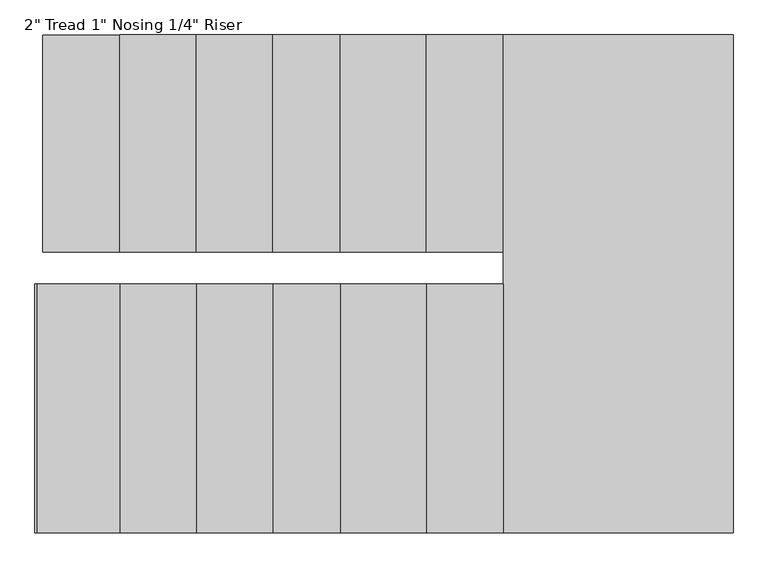
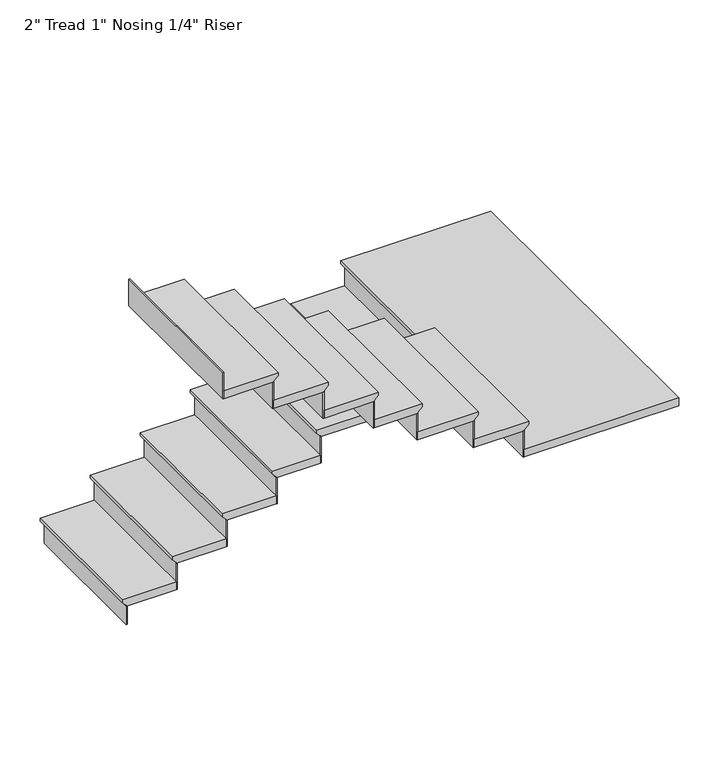
"""IFC4 building model written with IfcOpenShell, lengths in millimetres: stair flight geometry."""

from ifc_helpers import new_model, si_unit, origin, place, context, project, spatial, faceted_brep, source, transform, mapped, element, save


def stair_flight_0b56c5f1(model_context):
    return source(origin(), model_context, "Body", "Brep", [
        faceted_brep([(-879.540747, -2928.9064015, 150.2833333), (-879.540747, -2928.9064015, 169.3333333), (-879.540747, -2065.3064015, 169.3333333), (-879.540747, -2065.3064015, 150.2833333), (-854.140747, -2928.9064015, 124.8833333), (-854.140747, -2065.3064015, 124.8833333), (-549.340747, -2928.9064015, 169.3333333), (-549.340747, -2065.3064015, 169.3333333), (-854.140747, -2065.3064015, 118.5333333), (-549.340747, -2065.3064015, 118.5333333), (-549.340747, -2928.9064015, 118.5333333), (-854.140747, -2928.9064015, 118.5333333)], [[[0, 1, 2, 3]], [[4, 0, 3, 5]], [[2, 1, 6, 7]], [[8, 9, 10, 11]], [[2, 7, 9, 8, 5, 3]], [[8, 11, 4, 5]], [[6, 1, 0, 4, 11, 10]], [[7, 6, 10, 9]]]),
        faceted_brep([(-854.140747, -2928.9064015, 118.5333333), (-854.140747, -2928.9064015, 0.0), (-847.790747, -2928.9064015, 0.0), (-847.790747, -2928.9064015, 118.5333333), (-854.140747, -2065.3064015, 118.5333333), (-847.790747, -2065.3064015, 118.5333333), (-847.790747, -2065.3064015, 0.0), (-854.140747, -2065.3064015, 0.0)], [[[0, 1, 2, 3]], [[4, 5, 6, 7]], [[1, 0, 4, 7]], [[2, 1, 7, 6]], [[3, 2, 6, 5]], [[0, 3, 5, 4]]]),
        faceted_brep([(-549.340747, -2928.9064015, 287.8666667), (-549.340747, -2928.9064015, 118.5333333), (-542.990747, -2928.9064015, 118.5333333), (-542.990747, -2928.9064015, 287.8666667), (-549.340747, -2065.3064015, 287.8666667), (-542.990747, -2065.3064015, 287.8666667), (-542.990747, -2065.3064015, 118.5333333), (-549.340747, -2065.3064015, 118.5333333)], [[[0, 1, 2, 3]], [[4, 5, 6, 7]], [[1, 0, 4, 7]], [[2, 1, 7, 6]], [[3, 2, 6, 5]], [[0, 3, 5, 4]]]),
        faceted_brep([(-574.740747, -2065.3064015, 338.6666667), (-574.740747, -2928.9064015, 338.6666667), (-244.540747, -2928.9064015, 338.6666667), (-244.540747, -2065.3064015, 338.6666667), (-549.340747, -2065.3064015, 287.8666667), (-244.540747, -2065.3064015, 287.8666667), (-244.540747, -2928.9064015, 287.8666667), (-549.340747, -2928.9064015, 287.8666667), (-549.340747, -2065.3064015, 294.2166667), (-574.740747, -2065.3064015, 319.6166667), (-549.340747, -2928.9064015, 294.2166667), (-574.740747, -2928.9064015, 319.6166667)], [[[0, 1, 2, 3]], [[4, 5, 6, 7]], [[0, 3, 5, 4, 8, 9]], [[4, 7, 10, 8]], [[2, 1, 11, 10, 7, 6]], [[3, 2, 6, 5]], [[11, 1, 0, 9]], [[10, 11, 9, 8]]]),
        faceted_brep([(-244.540747, -2928.9064015, 457.2), (-244.540747, -2928.9064015, 287.8666667), (-238.190747, -2928.9064015, 287.8666667), (-238.190747, -2928.9064015, 457.2), (-244.540747, -2065.3064015, 457.2), (-238.190747, -2065.3064015, 457.2), (-238.190747, -2065.3064015, 287.8666667), (-244.540747, -2065.3064015, 287.8666667)], [[[0, 1, 2, 3]], [[4, 5, 6, 7]], [[1, 0, 4, 7]], [[2, 1, 7, 6]], [[3, 2, 6, 5]], [[0, 3, 5, 4]]]),
        faceted_brep([(-269.940747, -2065.3064015, 508.0), (-269.940747, -2928.9064015, 508.0), (60.259253, -2928.9064015, 508.0), (60.259253, -2065.3064015, 508.0), (-244.540747, -2065.3064015, 457.2), (60.259253, -2065.3064015, 457.2), (60.259253, -2928.9064015, 457.2), (-244.540747, -2928.9064015, 457.2), (-244.540747, -2065.3064015, 463.55), (-269.940747, -2065.3064015, 488.95), (-244.540747, -2928.9064015, 463.55), (-269.940747, -2928.9064015, 488.95)], [[[0, 1, 2, 3]], [[4, 5, 6, 7]], [[0, 3, 5, 4, 8, 9]], [[4, 7, 10, 8]], [[2, 1, 11, 10, 7, 6]], [[3, 2, 6, 5]], [[11, 1, 0, 9]], [[10, 11, 9, 8]]]),
        faceted_brep([(60.259253, -2928.9064015, 626.5333333), (60.259253, -2928.9064015, 457.2), (66.609253, -2928.9064015, 457.2), (66.609253, -2928.9064015, 626.5333333), (60.259253, -2065.3064015, 626.5333333), (66.609253, -2065.3064015, 626.5333333), (66.609253, -2065.3064015, 457.2), (60.259253, -2065.3064015, 457.2)], [[[0, 1, 2, 3]], [[4, 5, 6, 7]], [[1, 0, 4, 7]], [[2, 1, 7, 6]], [[3, 2, 6, 5]], [[0, 3, 5, 4]]]),
        faceted_brep([(34.859253, -2065.3064015, 677.3333333), (34.859253, -2928.9064015, 677.3333333), (326.959253, -2928.9064015, 677.3333333), (326.959253, -2065.3064015, 677.3333333), (60.259253, -2065.3064015, 626.5333333), (326.959253, -2065.3064015, 626.5333333), (326.959253, -2928.9064015, 626.5333333), (60.259253, -2928.9064015, 626.5333333), (60.259253, -2065.3064015, 632.8833333), (34.859253, -2065.3064015, 658.2833333), (60.259253, -2928.9064015, 632.8833333), (34.859253, -2928.9064015, 658.2833333)], [[[0, 1, 2, 3]], [[4, 5, 6, 7]], [[0, 3, 5, 4, 8, 9]], [[4, 7, 10, 8]], [[2, 1, 11, 10, 7, 6]], [[3, 2, 6, 5]], [[11, 1, 0, 9]], [[10, 11, 9, 8]]]),
        faceted_brep([(326.959253, -2928.9064015, 795.8666667), (326.959253, -2928.9064015, 626.5333333), (333.309253, -2928.9064015, 626.5333333), (333.309253, -2928.9064015, 795.8666667), (326.959253, -2065.3064015, 795.8666667), (333.309253, -2065.3064015, 795.8666667), (333.309253, -2065.3064015, 626.5333333), (326.959253, -2065.3064015, 626.5333333)], [[[0, 1, 2, 3]], [[4, 5, 6, 7]], [[1, 0, 4, 7]], [[2, 1, 7, 6]], [[3, 2, 6, 5]], [[0, 3, 5, 4]]]),
        faceted_brep([(301.559253, -2065.3064015, 846.6666667), (301.559253, -2928.9064015, 846.6666667), (669.859253, -2928.9064015, 846.6666667), (669.859253, -2065.3064015, 846.6666667), (326.959253, -2065.3064015, 795.8666667), (669.859253, -2065.3064015, 795.8666667), (669.859253, -2928.9064015, 795.8666667), (326.959253, -2928.9064015, 795.8666667), (326.959253, -2065.3064015, 802.2166667), (301.559253, -2065.3064015, 827.6166667), (326.959253, -2928.9064015, 802.2166667), (301.559253, -2928.9064015, 827.6166667)], [[[0, 1, 2, 3]], [[4, 5, 6, 7]], [[0, 3, 5, 4, 8, 9]], [[4, 7, 10, 8]], [[2, 1, 11, 10, 7, 6]], [[3, 2, 6, 5]], [[11, 1, 0, 9]], [[10, 11, 9, 8]]]),
        faceted_brep([(669.859253, -2928.9064015, 965.2), (669.859253, -2928.9064015, 795.8666667), (676.209253, -2928.9064015, 795.8666667), (676.209253, -2928.9064015, 965.2), (669.859253, -2065.3064015, 965.2), (676.209253, -2065.3064015, 965.2), (676.209253, -2065.3064015, 795.8666667), (669.859253, -2065.3064015, 795.8666667)], [[[0, 1, 2, 3]], [[4, 5, 6, 7]], [[1, 0, 4, 7]], [[2, 1, 7, 6]], [[3, 2, 6, 5]], [[0, 3, 5, 4]]]),
        faceted_brep([(644.459253, -2065.3064015, 1016.0), (644.459253, -2928.9064015, 1016.0), (974.659253, -2928.9064015, 1016.0), (974.659253, -2065.3064015, 1016.0), (669.859253, -2065.3064015, 965.2), (974.659253, -2065.3064015, 965.2), (974.659253, -2928.9064015, 965.2), (669.859253, -2928.9064015, 965.2), (669.859253, -2065.3064015, 971.55), (644.459253, -2065.3064015, 996.95), (669.859253, -2928.9064015, 971.55), (644.459253, -2928.9064015, 996.95)], [[[0, 1, 2, 3]], [[4, 5, 6, 7]], [[0, 3, 5, 4, 8, 9]], [[4, 7, 10, 8]], [[2, 1, 11, 10, 7, 6]], [[3, 2, 6, 5]], [[11, 1, 0, 9]], [[10, 11, 9, 8]]]),
        faceted_brep([(974.659253, -2928.9064015, 1134.5333333), (974.659253, -2928.9064015, 965.2), (981.009253, -2928.9064015, 965.2), (981.009253, -2928.9064015, 1134.5333333), (974.659253, -2065.3064015, 1134.5333333), (981.009253, -2065.3064015, 1134.5333333), (981.009253, -2065.3064015, 965.2), (974.659253, -2065.3064015, 965.2)], [[[0, 1, 2, 3]], [[4, 5, 6, 7]], [[1, 0, 4, 7]], [[2, 1, 7, 6]], [[3, 2, 6, 5]], [[0, 3, 5, 4]]]),
        faceted_brep([(923.859253, -4046.5064015, 1185.3333333), (1863.659253, -4046.5064015, 1185.3333333), (1863.659253, -2065.3064015, 1185.3333333), (949.259253, -2065.3064015, 1185.3333333), (949.259253, -3055.9064015, 1185.3333333), (923.859253, -3055.9064015, 1185.3333333), (1863.659253, -4046.5064015, 1134.5333333), (923.859253, -4046.5064015, 1134.5333333), (923.859253, -3055.9064015, 1134.5333333), (949.259253, -3055.9064015, 1134.5333333), (949.259253, -2928.9064015, 1134.5333333), (974.659253, -2928.9064015, 1134.5333333), (974.659253, -2065.3064015, 1134.5333333), (1863.659253, -2065.3064015, 1134.5333333), (974.659253, -2065.3064015, 1140.8833333), (949.259253, -2065.3064015, 1166.2833333), (974.659253, -2928.9064015, 1140.8833333), (949.259253, -2928.9064015, 1166.2833333)], [[[0, 1, 2, 3, 4, 5]], [[6, 7, 8, 9, 10, 11, 12, 13]], [[1, 0, 7, 6]], [[2, 1, 6, 13]], [[3, 2, 13, 12, 14, 15]], [[12, 11, 16, 14]], [[11, 10, 17, 16]], [[4, 3, 15, 17, 10, 9]], [[5, 4, 9, 8]], [[0, 5, 8, 7]], [[15, 14, 16, 17]]]),
        faceted_brep([(923.859253, -3055.9064015, 1303.8666667), (923.859253, -3055.9064015, 1134.5333333), (917.509253, -3055.9064015, 1134.5333333), (917.509253, -3055.9064015, 1303.8666667), (923.859253, -4046.5064015, 1303.8666667), (917.509253, -4046.5064015, 1303.8666667), (917.509253, -4046.5064015, 1134.5333333), (923.859253, -4046.5064015, 1134.5333333)], [[[0, 1, 2, 3]], [[4, 5, 6, 7]], [[1, 0, 4, 7]], [[2, 1, 7, 6]], [[3, 2, 6, 5]], [[0, 3, 5, 4]]]),
        faceted_brep([(949.259253, -4046.5064015, 1354.6666667), (949.259253, -3055.9064015, 1354.6666667), (619.059253, -3055.9064015, 1354.6666667), (619.059253, -4046.5064015, 1354.6666667), (923.859253, -4046.5064015, 1303.8666667), (619.059253, -4046.5064015, 1303.8666667), (619.059253, -3055.9064015, 1303.8666667), (923.859253, -3055.9064015, 1303.8666667), (923.859253, -4046.5064015, 1310.2166667), (949.259253, -4046.5064015, 1335.6166667), (923.859253, -3055.9064015, 1310.2166667), (949.259253, -3055.9064015, 1335.6166667)], [[[0, 1, 2, 3]], [[4, 5, 6, 7]], [[0, 3, 5, 4, 8, 9]], [[4, 7, 10, 8]], [[2, 1, 11, 10, 7, 6]], [[3, 2, 6, 5]], [[11, 1, 0, 9]], [[10, 11, 9, 8]]]),
        faceted_brep([(619.059253, -3055.9064015, 1473.2), (619.059253, -3055.9064015, 1303.8666667), (612.709253, -3055.9064015, 1303.8666667), (612.709253, -3055.9064015, 1473.2), (619.059253, -4046.5064015, 1473.2), (612.709253, -4046.5064015, 1473.2), (612.709253, -4046.5064015, 1303.8666667), (619.059253, -4046.5064015, 1303.8666667)], [[[0, 1, 2, 3]], [[4, 5, 6, 7]], [[1, 0, 4, 7]], [[2, 1, 7, 6]], [[3, 2, 6, 5]], [[0, 3, 5, 4]]]),
        faceted_brep([(644.459253, -4046.5064015, 1524.0), (644.459253, -3055.9064015, 1524.0), (276.159253, -3055.9064015, 1524.0), (276.159253, -4046.5064015, 1524.0), (619.059253, -4046.5064015, 1473.2), (276.159253, -4046.5064015, 1473.2), (276.159253, -3055.9064015, 1473.2), (619.059253, -3055.9064015, 1473.2), (619.059253, -4046.5064015, 1479.55), (644.459253, -4046.5064015, 1504.95), (619.059253, -3055.9064015, 1479.55), (644.459253, -3055.9064015, 1504.95)], [[[0, 1, 2, 3]], [[4, 5, 6, 7]], [[0, 3, 5, 4, 8, 9]], [[4, 7, 10, 8]], [[2, 1, 11, 10, 7, 6]], [[3, 2, 6, 5]], [[11, 1, 0, 9]], [[10, 11, 9, 8]]]),
        faceted_brep([(276.159253, -3055.9064015, 1642.5333333), (276.159253, -3055.9064015, 1473.2), (269.809253, -3055.9064015, 1473.2), (269.809253, -3055.9064015, 1642.5333333), (276.159253, -4046.5064015, 1642.5333333), (269.809253, -4046.5064015, 1642.5333333), (269.809253, -4046.5064015, 1473.2), (276.159253, -4046.5064015, 1473.2)], [[[0, 1, 2, 3]], [[4, 5, 6, 7]], [[1, 0, 4, 7]], [[2, 1, 7, 6]], [[3, 2, 6, 5]], [[0, 3, 5, 4]]]),
        faceted_brep([(301.559253, -4046.5064015, 1693.3333333), (301.559253, -3055.9064015, 1693.3333333), (9.459253, -3055.9064015, 1693.3333333), (9.459253, -4046.5064015, 1693.3333333), (276.159253, -4046.5064015, 1642.5333333), (9.459253, -4046.5064015, 1642.5333333), (9.459253, -3055.9064015, 1642.5333333), (276.159253, -3055.9064015, 1642.5333333), (276.159253, -4046.5064015, 1648.8833333), (301.559253, -4046.5064015, 1674.2833333), (276.159253, -3055.9064015, 1648.8833333), (301.559253, -3055.9064015, 1674.2833333)], [[[0, 1, 2, 3]], [[4, 5, 6, 7]], [[0, 3, 5, 4, 8, 9]], [[4, 7, 10, 8]], [[2, 1, 11, 10, 7, 6]], [[3, 2, 6, 5]], [[11, 1, 0, 9]], [[10, 11, 9, 8]]]),
        faceted_brep([(9.459253, -3055.9064015, 1811.8666667), (9.459253, -3055.9064015, 1642.5333333), (3.109253, -3055.9064015, 1642.5333333), (3.109253, -3055.9064015, 1811.8666667), (9.459253, -4046.5064015, 1811.8666667), (3.109253, -4046.5064015, 1811.8666667), (3.109253, -4046.5064015, 1642.5333333), (9.459253, -4046.5064015, 1642.5333333)], [[[0, 1, 2, 3]], [[4, 5, 6, 7]], [[1, 0, 4, 7]], [[2, 1, 7, 6]], [[3, 2, 6, 5]], [[0, 3, 5, 4]]]),
        faceted_brep([(34.859253, -4046.5064015, 1862.6666667), (34.859253, -3055.9064015, 1862.6666667), (-295.340747, -3055.9064015, 1862.6666667), (-295.340747, -4046.5064015, 1862.6666667), (9.459253, -4046.5064015, 1811.8666667), (-295.340747, -4046.5064015, 1811.8666667), (-295.340747, -3055.9064015, 1811.8666667), (9.459253, -3055.9064015, 1811.8666667), (9.459253, -4046.5064015, 1818.2166667), (34.859253, -4046.5064015, 1843.6166667), (9.459253, -3055.9064015, 1818.2166667), (34.859253, -3055.9064015, 1843.6166667)], [[[0, 1, 2, 3]], [[4, 5, 6, 7]], [[0, 3, 5, 4, 8, 9]], [[4, 7, 10, 8]], [[2, 1, 11, 10, 7, 6]], [[3, 2, 6, 5]], [[11, 1, 0, 9]], [[10, 11, 9, 8]]]),
        faceted_brep([(-295.340747, -3055.9064015, 1981.2), (-295.340747, -3055.9064015, 1811.8666667), (-301.690747, -3055.9064015, 1811.8666667), (-301.690747, -3055.9064015, 1981.2), (-295.340747, -4046.5064015, 1981.2), (-301.690747, -4046.5064015, 1981.2), (-301.690747, -4046.5064015, 1811.8666667), (-295.340747, -4046.5064015, 1811.8666667)], [[[0, 1, 2, 3]], [[4, 5, 6, 7]], [[1, 0, 4, 7]], [[2, 1, 7, 6]], [[3, 2, 6, 5]], [[0, 3, 5, 4]]]),
        faceted_brep([(-269.940747, -4046.5064015, 2032.0), (-269.940747, -3055.9064015, 2032.0), (-600.140747, -3055.9064015, 2032.0), (-600.140747, -4046.5064015, 2032.0), (-295.340747, -4046.5064015, 1981.2), (-600.140747, -4046.5064015, 1981.2), (-600.140747, -3055.9064015, 1981.2), (-295.340747, -3055.9064015, 1981.2), (-295.340747, -4046.5064015, 1987.55), (-269.940747, -4046.5064015, 2012.95), (-295.340747, -3055.9064015, 1987.55), (-269.940747, -3055.9064015, 2012.95)], [[[0, 1, 2, 3]], [[4, 5, 6, 7]], [[0, 3, 5, 4, 8, 9]], [[4, 7, 10, 8]], [[2, 1, 11, 10, 7, 6]], [[3, 2, 6, 5]], [[11, 1, 0, 9]], [[10, 11, 9, 8]]]),
        faceted_brep([(-600.140747, -3055.9064015, 2150.5333333), (-600.140747, -3055.9064015, 1981.2), (-606.490747, -3055.9064015, 1981.2), (-606.490747, -3055.9064015, 2150.5333333), (-600.140747, -4046.5064015, 2150.5333333), (-606.490747, -4046.5064015, 2150.5333333), (-606.490747, -4046.5064015, 1981.2), (-600.140747, -4046.5064015, 1981.2)], [[[0, 1, 2, 3]], [[4, 5, 6, 7]], [[1, 0, 4, 7]], [[2, 1, 7, 6]], [[3, 2, 6, 5]], [[0, 3, 5, 4]]]),
        faceted_brep([(-904.940747, -3055.9064015, 2319.8666667), (-904.940747, -3055.9064015, 2150.5333333), (-911.290747, -3055.9064015, 2150.5333333), (-911.290747, -3055.9064015, 2319.8666667), (-904.940747, -4046.5064015, 2319.8666667), (-911.290747, -4046.5064015, 2319.8666667), (-911.290747, -4046.5064015, 2150.5333333), (-904.940747, -4046.5064015, 2150.5333333)], [[[0, 1, 2, 3]], [[4, 5, 6, 7]], [[1, 0, 4, 7]], [[2, 1, 7, 6]], [[3, 2, 6, 5]], [[0, 3, 5, 4]]]),
        faceted_brep([(-574.740747, -4046.5064015, 2201.3333333), (-574.740747, -3055.9064015, 2201.3333333), (-904.940747, -3055.9064015, 2201.3333333), (-904.940747, -4046.5064015, 2201.3333333), (-600.140747, -4046.5064015, 2150.5333333), (-904.940747, -4046.5064015, 2150.5333333), (-904.940747, -3055.9064015, 2150.5333333), (-600.140747, -3055.9064015, 2150.5333333), (-600.140747, -4046.5064015, 2156.8833333), (-574.740747, -4046.5064015, 2182.2833333), (-600.140747, -3055.9064015, 2156.8833333), (-574.740747, -3055.9064015, 2182.2833333)], [[[0, 1, 2, 3]], [[4, 5, 6, 7]], [[0, 3, 5, 4, 8, 9]], [[4, 7, 10, 8]], [[2, 1, 11, 10, 7, 6]], [[3, 2, 6, 5]], [[11, 1, 0, 9]], [[10, 11, 9, 8]]]),
    ])


if __name__ == "__main__":
    model = new_model("IFC4")
    model_context = context("Model", 3, world=origin())
    ifc_project = project(units=[si_unit("LENGTHUNIT", "METRE", prefix="MILLI")], contexts=[model_context])
    site = spatial("IfcSite", under=ifc_project)
    building = spatial("IfcBuilding", under=site)
    placement = place(None, origin())
    stair_flight_shape = stair_flight_0b56c5f1(model_context)
    element("IfcStairFlight", 1, ObjectType="2\" Tread 1\" Nosing 1/4\" Riser", at=placement, inside=building, context=model_context, shape_type="MappedRepresentation", body=[
        mapped(stair_flight_shape, transform((0.0, 0.0, 0.0), x_axis=(1.0, 0.0, 0.0), y_axis=(0.0, 1.0, 0.0), z_axis=(0.0, 0.0, 1.0))),
    ])
    save(model, "model.ifc")
